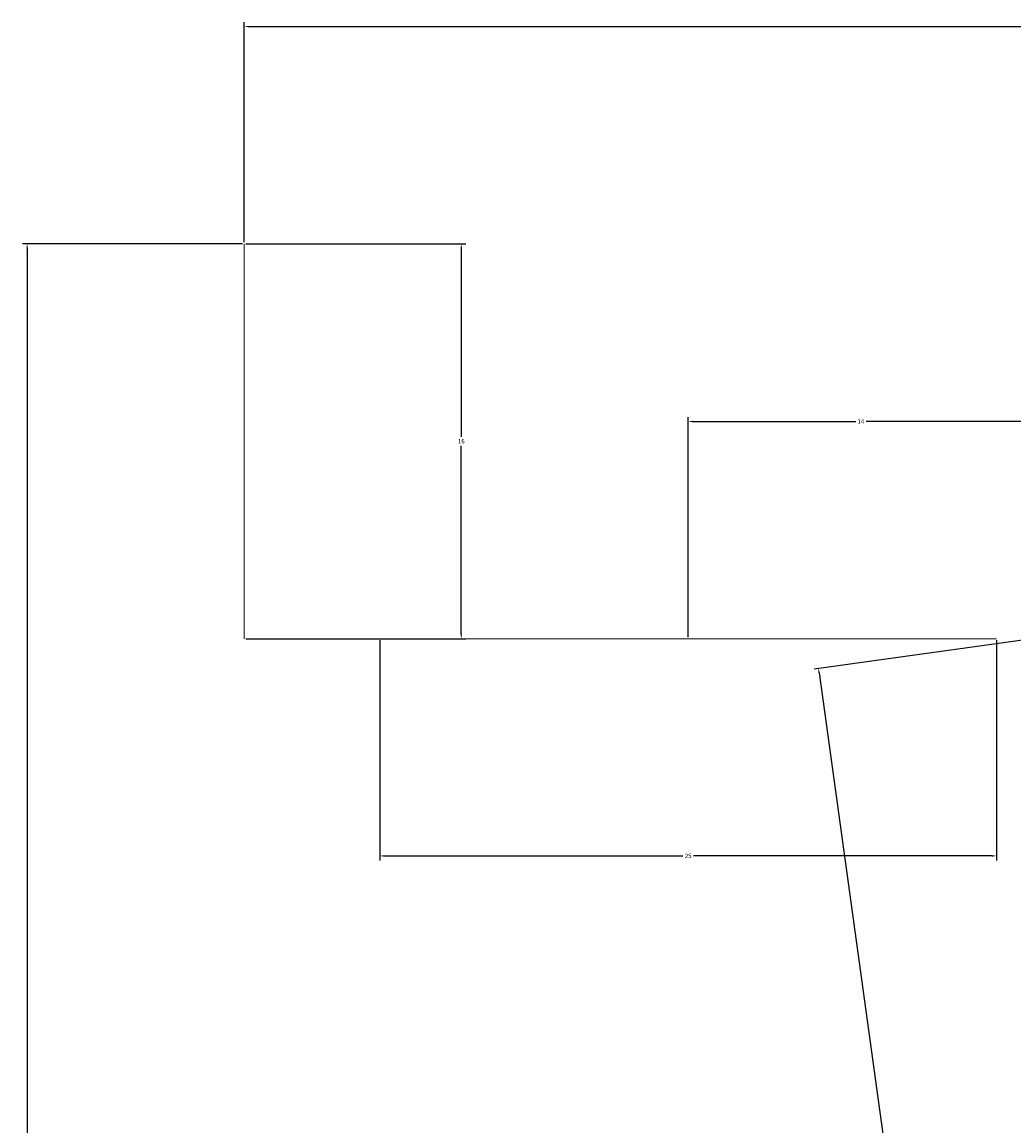
# Model space of a CAD drawing. Units: millimetres. Extents: x -9 to 135, y -119 to 27.
# Tile 4 of 12: x -9 to 31, y -18 to 27. Entities that reach past the tile are written whole.
import ezdxf

# ---------------------------------------------------------------- set-up
doc = ezdxf.new("R2010")
doc.units = ezdxf.units.MM
doc.layers.add('M-CONS', color=8, linetype='Continuous', lineweight=18)
doc.layers.add('M-DIMS', color=2, linetype='Continuous', lineweight=18)
doc.styles.get("Standard").update_dxf_attribs({"font": 'arial.ttf'})
doc.dimstyles.get("Standard").update_dxf_attribs({"dimtxt": 0.18, "dimasz": 0.18, "dimexe": 0.18, "dimexo": 0.0625, "dimgap": 0.09, "dimtad": 0, "dimtih": 1, "dimtoh": 1, "dimdec": 4, "dimzin": 0, "dimdsep": 46, "dimtxsty": 'Standard', "dimcen": 0.09, "dimadec": 0, "dimazin": 0, "dimtfac": 1, "dimtdec": 4, "dimtofl": 0, "dimtmove": 0, "dimatfit": 3, "dimfxl": 1, "dimtolj": 1, "dimtzin": 0, "dimarcsym": 0})

# ---------------------------------------------------------------- blocks, each defined once
blk = doc.blocks.new('BOSS-PROFILE-D25-BORE10')
at = {"extrusion": (0, -1, 0)}
for radius in [12.5, 5]:
    blk.add_circle((12.5, 101.129, 0), radius, dxfattribs=at)
blk = doc.blocks.new('*D2')
at = {"layer": 'Defpoints', "color": 0, "transparency": 16777216}
for p in [(126, 26.533), (0, 17.733), (126, 1.733)]:
    blk.add_point(p, dxfattribs=at)
at = {"layer": 'M-DIMS', "color": 0, "lineweight": -2, "transparency": 16777216}
for p, q in [((0, 17.796), (0, 26.713)), ((0.18, 26.533), (62.72, 26.533)), ((125.82, 26.533), (63.28, 26.533)), ((126, 1.796), (126, 26.713))]:
    blk.add_line(p, q, dxfattribs=at)
at = {"layer": 'M-DIMS', "color": 0, "transparency": 16777216}
for points in [[(0.18, 26.563), (0.18, 26.503), (0, 26.533)], [(125.82, 26.563), (125.82, 26.503), (126, 26.533)]]:
    blk.add_solid(points, dxfattribs=at)
at = {"layer": 'M-DIMS', "color": 0, "transparency": 16777216, "insert": (63, 26.533), "char_height": 0.18, "attachment_point": 5}
blk.add_mtext('\\A1;126', dxfattribs=at)
blk = doc.blocks.new('*D3')
at = {"layer": 'Defpoints', "color": 0, "transparency": 16777216}
for p in [(0, 17.733), (-8.8, -110.267), (63, -110.267)]:
    blk.add_point(p, dxfattribs=at)
at = {"layer": 'M-DIMS', "color": 0, "lineweight": -2, "transparency": 16777216}
for p, q in [((-0.062, 17.733), (-8.98, 17.733)), ((-8.8, 17.553), (-8.8, -46.085)), ((-8.8, -110.087), (-8.8, -46.449)), ((62.938, -110.267), (-8.98, -110.267))]:
    blk.add_line(p, q, dxfattribs=at)
at = {"layer": 'M-DIMS', "color": 0, "transparency": 16777216}
for points in [[(-8.83, 17.553), (-8.77, 17.553), (-8.8, 17.733)], [(-8.83, -110.087), (-8.77, -110.087), (-8.8, -110.267)]]:
    blk.add_solid(points, dxfattribs=at)
at = {"layer": 'M-DIMS', "color": 0, "transparency": 16777216, "insert": (-8.8, -46.267), "char_height": 0.18, "attachment_point": 5}
blk.add_mtext('\\A1;128', dxfattribs=at)
blk = doc.blocks.new('*D4')
at = {"layer": 'Defpoints', "color": 0, "transparency": 16777216}
for p in [(0, 17.733), (0, 1.733), (8.8, 1.733)]:
    blk.add_point(p, dxfattribs=at)
at = {"layer": 'M-DIMS', "color": 0, "lineweight": -2, "transparency": 16777216}
for p, q in [((0.062, 17.733), (8.98, 17.733)), ((8.8, 17.553), (8.8, 9.915)), ((8.8, 1.913), (8.8, 9.551)), ((0.062, 1.733), (8.98, 1.733))]:
    blk.add_line(p, q, dxfattribs=at)
at = {"layer": 'M-DIMS', "color": 0, "transparency": 16777216}
for points in [[(8.77, 17.553), (8.83, 17.553), (8.8, 17.733)], [(8.77, 1.913), (8.83, 1.913), (8.8, 1.733)]]:
    blk.add_solid(points, dxfattribs=at)
at = {"layer": 'M-DIMS', "color": 0, "transparency": 16777216, "insert": (8.8, 9.733), "char_height": 0.18, "attachment_point": 5}
blk.add_mtext('\\A1;16', dxfattribs=at)
blk = doc.blocks.new('*D5')
at = {"layer": 'Defpoints', "color": 0, "transparency": 16777216}
for p in [(32, 10.533), (18, 1.733), (32, 1.733)]:
    blk.add_point(p, dxfattribs=at)
at = {"layer": 'M-DIMS', "color": 0, "lineweight": -2, "transparency": 16777216}
for p, q in [((18, 1.796), (18, 10.713)), ((18.18, 10.533), (24.79, 10.533)), ((31.82, 10.533), (25.21, 10.533)), ((32, 1.796), (32, 10.713))]:
    blk.add_line(p, q, dxfattribs=at)
at = {"layer": 'M-DIMS', "color": 0, "transparency": 16777216}
for points in [[(18.18, 10.563), (18.18, 10.503), (18, 10.533)], [(31.82, 10.563), (31.82, 10.503), (32, 10.533)]]:
    blk.add_solid(points, dxfattribs=at)
at = {"layer": 'M-DIMS', "color": 0, "transparency": 16777216, "insert": (25, 10.533), "char_height": 0.18, "attachment_point": 5}
blk.add_mtext('\\A1;14', dxfattribs=at)
blk = doc.blocks.new('*D8')
at = {"layer": 'Defpoints', "color": 0, "transparency": 16777216}
for p in [(5.5, 1.733), (30.5, 1.733), (5.5, -7.067)]:
    blk.add_point(p, dxfattribs=at)
at = {"layer": 'M-DIMS', "color": 0, "lineweight": -2, "transparency": 16777216}
for p, q in [((5.5, 1.671), (5.5, -7.247)), ((30.5, 1.671), (30.5, -7.247)), ((5.68, -7.067), (17.779, -7.067)), ((30.32, -7.067), (18.221, -7.067))]:
    blk.add_line(p, q, dxfattribs=at)
at = {"layer": 'M-DIMS', "color": 0, "transparency": 16777216}
for points in [[(5.68, -7.037), (5.68, -7.097), (5.5, -7.067)], [(30.32, -7.037), (30.32, -7.097), (30.5, -7.067)]]:
    blk.add_solid(points, dxfattribs=at)
at = {"layer": 'M-DIMS', "color": 0, "transparency": 16777216, "insert": (18, -7.067), "char_height": 0.18, "attachment_point": 5}
blk.add_mtext('\\A1;25', dxfattribs=at)
blk = doc.blocks.new('*D14')
at = {"layer": 'Defpoints', "color": 0, "transparency": 16777216}
for p in [(32, 1.733), (23.283, 0.528), (45, -92.267)]:
    blk.add_point(p, dxfattribs=at)
at = {"layer": 'M-DIMS', "color": 0, "lineweight": -2, "transparency": 16777216}
for p, q in [((31.938, 1.725), (23.105, 0.503)), ((23.308, 0.349), (29.758, -46.29)), ((36.258, -93.294), (29.808, -46.654)), ((44.938, -92.275), (36.105, -93.497))]:
    blk.add_line(p, q, dxfattribs=at)
at = {"layer": 'M-DIMS', "color": 0, "transparency": 16777216}
for points in [[(23.337, 0.353), (23.278, 0.345), (23.283, 0.528)], [(36.288, -93.29), (36.229, -93.298), (36.283, -93.472)]]:
    blk.add_solid(points, dxfattribs=at)
at = {"layer": 'M-DIMS', "color": 0, "transparency": 16777216, "insert": (29.783, -46.472), "char_height": 0.18, "attachment_point": 5}
blk.add_mtext('\\A1;94.9', dxfattribs=at)

msp = doc.modelspace()

# ---------------------------------------------------------------- linework, layer by layer
at = {"layer": 'M-CONS', "extrusion": (1, 0, 0)}
msp.add_lwpolyline([(17.733, 131.129), (17.733, 121.129), (14.733, 121.129), (14.733, 81.129), (17.733, 81.129), (17.733, 71.129), (1.733, 71.129), (1.733, 131.129)], close=True, dxfattribs=at)

# ---------------------------------------------------------------- block references
at = {"layer": 'M-CONS'}
msp.add_blockref('BOSS-PROFILE-D25-BORE10', (5.5, 1.733), dxfattribs=at)

# ---------------------------------------------------------------- dimensions: what is measured, and where the dimension line sits
at = {"layer": 'M-DIMS'}
for base, p1, p2, picture, middle in [((126, 26.533), (0, 17.733), (126, 1.733), '*D2', (63, 26.533)), ((32, 10.533), (18, 1.733), (32, 1.733), '*D5', (25, 10.533))]:
    dim = msp.add_linear_dim(base=base, p1=p1, p2=p2, dimstyle='Standard', override={"dimdec": 0, "dimlfac": 1, "dimrnd": 0, "dimzin": 0, "dimdsep": 46, "dimlunit": 2}, dxfattribs=at)
    dim.commit()
    dim.dimension.update_dxf_attribs({"geometry": picture, "text_midpoint": middle})
for base, p1, p2, angle, override, picture, middle in [((-8.8, -110.267), (0, 17.733), (63, -110.267), 90, {"dimdec": 0, "dimlfac": 1, "dimrnd": 0, "dimzin": 0, "dimdsep": 46, "dimlunit": 2}, '*D3', (-8.8, -46.267)), ((8.8, 1.733), (0, 17.733), (0, 1.733), 270, {"dimdec": 0, "dimlfac": 1, "dimrnd": 0, "dimzin": 0, "dimdsep": 46, "dimlunit": 2}, '*D4', (8.8, 9.733)), ((5.5, -7.067), (30.5, 1.733), (5.5, 1.733), 180, {"dimdec": 0, "dimlfac": 1, "dimrnd": 0, "dimzin": 0, "dimdsep": 46, "dimlunit": 2}, '*D8', (18, -7.067)), ((23.283, 0.528), (45, -92.267), (32, 1.733), 97.8739, {"dimdec": 1, "dimlfac": 1, "dimrnd": 0, "dimzin": 0, "dimdsep": 46, "dimlunit": 2}, '*D14', (29.783, -46.472))]:
    dim = msp.add_linear_dim(base=base, p1=p1, p2=p2, angle=angle, dimstyle='Standard', override=override, dxfattribs=at)
    dim.commit()
    dim.dimension.update_dxf_attribs({"geometry": picture, "text_midpoint": middle})

doc.saveas('drawing.dxf')
